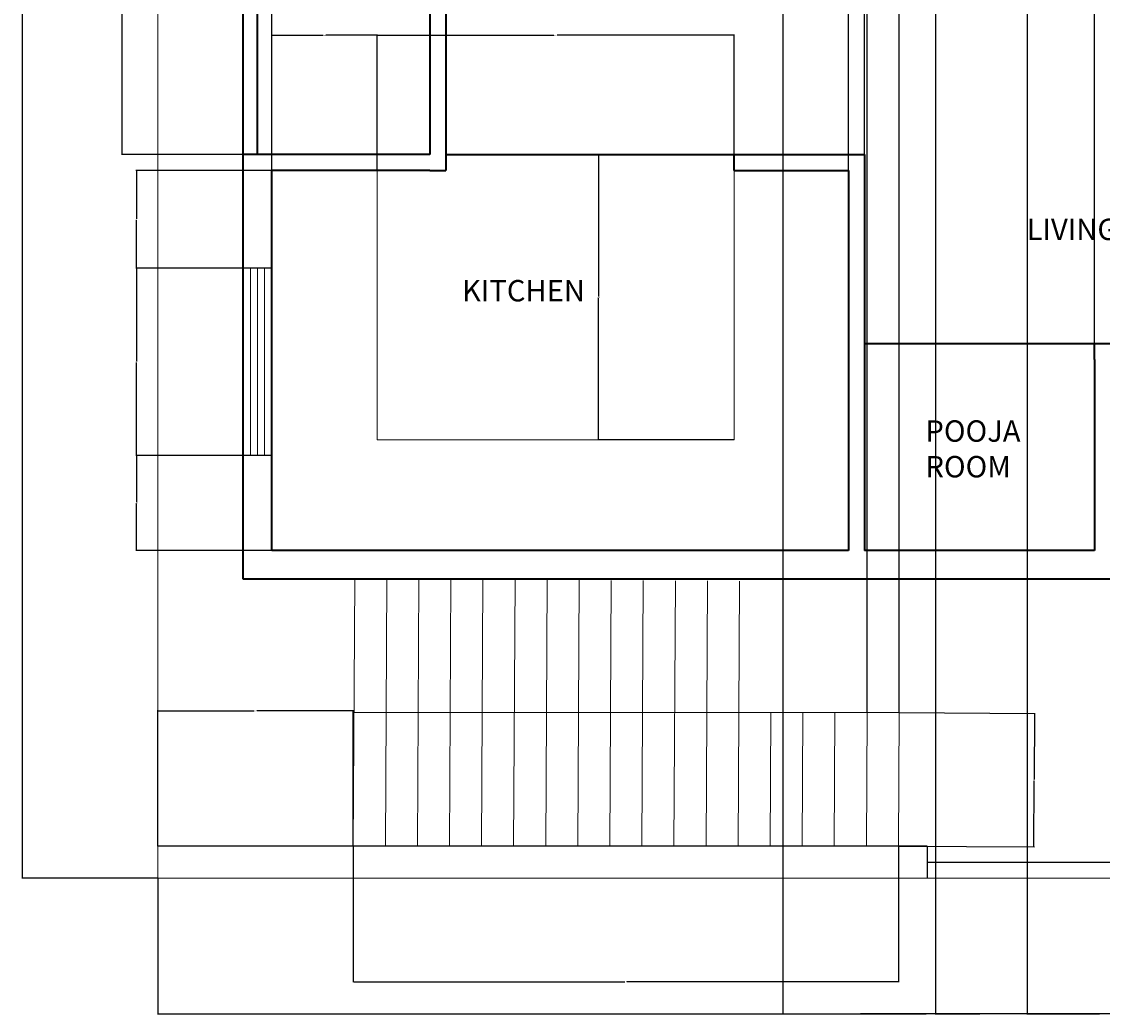
# Model space of a CAD drawing. Units: inches. Extents: x 4700 to 5209, y 8078 to 8754.
# Tile 1 of 5: x 4701 to 5004, y 8078 to 8356. Entities that reach past the tile are written whole.
import ezdxf

# ---------------------------------------------------------------- set-up
doc = ezdxf.new("R2010")
doc.units = ezdxf.units.IN
for name, color, linetype, lineweight in [('A-ANNO-DIMS', 2, 'Continuous', 18), ('A-AREA-IDEN', 7, 'Continuous', 18), ('A-FLOR', 7, 'Continuous', 25), ('A-FLOR-FIXT', 9, 'Continuous', 18), ('A-FLOR-STRS', 7, 'Continuous', 18), ('A-GLAZ', 4, 'Continuous', 18), ('A-WALL', 7, 'Continuous', 35), ('C-PROP', 8, 'Continuous', 18)]:
    doc.layers.add(name, color=color, linetype=linetype, lineweight=lineweight)
doc.styles.get("Standard").update_dxf_attribs({"font": 'arial.ttf'})
doc.dimstyles.get("Standard").update_dxf_attribs({"dimtxt": 0.18, "dimasz": 0.18, "dimexe": 0.18, "dimexo": 0.0625, "dimgap": 0.09, "dimtad": 0, "dimtih": 1, "dimtoh": 1, "dimdec": 4, "dimzin": 0, "dimdsep": 46, "dimtxsty": 'Standard', "dimcen": 0.09, "dimadec": 0, "dimazin": 0, "dimtfac": 1, "dimtdec": 4, "dimtofl": 0, "dimtmove": 0, "dimatfit": 3, "dimfxl": 1, "dimtolj": 1, "dimtzin": 0, "dimarcsym": 0})

# ---------------------------------------------------------------- blocks, each defined once
blk = doc.blocks.new('*D14')
at = {"layer": 'A-ANNO-DIMS', "color": 0, "lineweight": -2, "transparency": 16777216}
for p, q in [((4738.78, 8115.69), (4738.78, 8077.57)), ((5170.78, 8115.69), (5170.78, 8077.57)), ((4738.96, 8077.75), (4954.49, 8077.75)), ((5170.6, 8077.75), (4955.07, 8077.75))]:
    blk.add_line(p, q, dxfattribs=at)
at = {"layer": 'A-ANNO-DIMS', "color": 0, "transparency": 16777216}
for points in [[(4738.96, 8077.78), (4738.96, 8077.72), (4738.78, 8077.75)], [(5170.6, 8077.78), (5170.6, 8077.72), (5170.78, 8077.75)]]:
    blk.add_solid(points, dxfattribs=at)
at = {"layer": 'Defpoints', "color": 0, "transparency": 16777216}
for p in [(4738.78, 8115.75), (5170.78, 8115.75), (5170.78, 8077.75)]:
    blk.add_point(p, dxfattribs=at)
at = {"layer": 'A-ANNO-DIMS', "color": 0, "transparency": 16777216, "insert": (4954.78, 8077.75), "char_height": 0.18, "attachment_point": 5}
blk.add_mtext('\\A1;432', dxfattribs=at)
blk = doc.blocks.new('*D15')
at = {"layer": 'A-ANNO-DIMS', "color": 0, "lineweight": -2, "transparency": 16777216}
for p, q in [((4738.72, 8715.75), (4700.6, 8715.75)), ((4700.78, 8715.57), (4700.78, 8415.93)), ((4700.78, 8115.93), (4700.78, 8415.57)), ((4738.72, 8115.75), (4700.6, 8115.75))]:
    blk.add_line(p, q, dxfattribs=at)
at = {"layer": 'A-ANNO-DIMS', "color": 0, "transparency": 16777216}
for points in [[(4700.75, 8715.57), (4700.81, 8715.57), (4700.78, 8715.75)], [(4700.75, 8115.93), (4700.81, 8115.93), (4700.78, 8115.75)]]:
    blk.add_solid(points, dxfattribs=at)
at = {"layer": 'Defpoints', "color": 0, "transparency": 16777216}
for p in [(4700.78, 8715.75), (4738.78, 8715.75), (4738.78, 8115.75)]:
    blk.add_point(p, dxfattribs=at)
at = {"layer": 'A-ANNO-DIMS', "color": 0, "transparency": 16777216, "insert": (4700.78, 8415.75), "char_height": 0.18, "attachment_point": 5}
blk.add_mtext('\\A1;600', dxfattribs=at)
blk = doc.blocks.new('*D28')
at = {"layer": 'A-ANNO-DIMS', "color": 0, "lineweight": -2, "transparency": 16777216}
for p, q in [((4770.72, 8234.43), (4732.6, 8234.43)), ((4732.78, 8234.25), (4732.78, 8221.27)), ((4732.78, 8207.93), (4732.78, 8220.91)), ((4770.72, 8207.75), (4732.6, 8207.75))]:
    blk.add_line(p, q, dxfattribs=at)
at = {"layer": 'A-ANNO-DIMS', "color": 0, "transparency": 16777216}
for points in [[(4732.75, 8234.25), (4732.81, 8234.25), (4732.78, 8234.43)], [(4732.75, 8207.93), (4732.81, 8207.93), (4732.78, 8207.75)]]:
    blk.add_solid(points, dxfattribs=at)
at = {"layer": 'Defpoints', "color": 0, "transparency": 16777216}
for p in [(4732.78, 8234.43), (4770.78, 8234.43), (4770.78, 8207.75)]:
    blk.add_point(p, dxfattribs=at)
at = {"layer": 'A-ANNO-DIMS', "color": 0, "transparency": 16777216, "insert": (4732.78, 8221.09), "char_height": 0.18, "attachment_point": 5}
blk.add_mtext('\\A1;26.684', dxfattribs=at)
blk = doc.blocks.new('*D29')
at = {"layer": 'A-ANNO-DIMS', "color": 0, "lineweight": -2, "transparency": 16777216}
for p, q in [((4770.72, 8286.99), (4732.6, 8286.99)), ((4732.78, 8286.81), (4732.78, 8260.89)), ((4732.78, 8234.61), (4732.78, 8260.53)), ((4770.72, 8234.43), (4732.6, 8234.43))]:
    blk.add_line(p, q, dxfattribs=at)
at = {"layer": 'A-ANNO-DIMS', "color": 0, "transparency": 16777216}
for points in [[(4732.75, 8286.81), (4732.81, 8286.81), (4732.78, 8286.99)], [(4732.75, 8234.61), (4732.81, 8234.61), (4732.78, 8234.43)]]:
    blk.add_solid(points, dxfattribs=at)
at = {"layer": 'Defpoints', "color": 0, "transparency": 16777216}
for p in [(4732.78, 8286.99), (4770.78, 8286.99), (4770.78, 8234.43)]:
    blk.add_point(p, dxfattribs=at)
at = {"layer": 'A-ANNO-DIMS', "color": 0, "transparency": 16777216, "insert": (4732.78, 8260.71), "char_height": 0.18, "attachment_point": 5}
blk.add_mtext('\\A1;52.55', dxfattribs=at)
blk = doc.blocks.new('*D30')
at = {"layer": 'A-ANNO-DIMS', "color": 0, "lineweight": -2, "transparency": 16777216}
for p, q in [((4770.72, 8314.35), (4732.6, 8314.35)), ((4732.78, 8314.17), (4732.78, 8300.85)), ((4732.78, 8287.17), (4732.78, 8300.49)), ((4770.72, 8286.99), (4732.6, 8286.99))]:
    blk.add_line(p, q, dxfattribs=at)
at = {"layer": 'A-ANNO-DIMS', "color": 0, "transparency": 16777216}
for points in [[(4732.75, 8314.17), (4732.81, 8314.17), (4732.78, 8314.35)], [(4732.75, 8287.17), (4732.81, 8287.17), (4732.78, 8286.99)]]:
    blk.add_solid(points, dxfattribs=at)
at = {"layer": 'Defpoints', "color": 0, "transparency": 16777216}
for p in [(4732.78, 8314.35), (4770.78, 8314.35), (4770.78, 8286.99)]:
    blk.add_point(p, dxfattribs=at)
at = {"layer": 'A-ANNO-DIMS', "color": 0, "transparency": 16777216, "insert": (4732.78, 8300.67), "char_height": 0.18, "attachment_point": 5}
blk.add_mtext('\\A1;27.36', dxfattribs=at)
blk = doc.blocks.new('*D31')
at = {"layer": 'A-ANNO-DIMS', "color": 0, "lineweight": -2, "transparency": 16777216}
for p, q in [((4766.72, 8445.91), (4728.6, 8445.91)), ((4728.78, 8445.73), (4728.78, 8382.56)), ((4728.78, 8319.03), (4728.78, 8382.19)), ((4766.72, 8318.85), (4728.6, 8318.85))]:
    blk.add_line(p, q, dxfattribs=at)
at = {"layer": 'A-ANNO-DIMS', "color": 0, "transparency": 16777216}
for points in [[(4728.75, 8445.73), (4728.81, 8445.73), (4728.78, 8445.91)], [(4728.75, 8319.03), (4728.81, 8319.03), (4728.78, 8318.85)]]:
    blk.add_solid(points, dxfattribs=at)
at = {"layer": 'Defpoints', "color": 0, "transparency": 16777216}
for p in [(4728.78, 8445.91), (4766.78, 8445.91), (4766.78, 8318.85)]:
    blk.add_point(p, dxfattribs=at)
at = {"layer": 'A-ANNO-DIMS', "color": 0, "transparency": 16777216, "insert": (4728.78, 8382.38), "char_height": 0.18, "attachment_point": 5}
blk.add_mtext('\\A1;127.06', dxfattribs=at)
blk = doc.blocks.new('*D49')
at = {"layer": 'A-ANNO-DIMS', "color": 0, "lineweight": -2, "transparency": 16777216}
for p, q in [((4766.78, 8318.91), (4766.78, 8753.93)), ((4766.96, 8753.75), (4790.57, 8753.75)), ((4814.97, 8753.75), (4791.36, 8753.75)), ((4815.15, 8318.91), (4815.15, 8753.93))]:
    blk.add_line(p, q, dxfattribs=at)
at = {"layer": 'A-ANNO-DIMS', "color": 0, "transparency": 16777216}
for points in [[(4766.96, 8753.78), (4766.96, 8753.72), (4766.78, 8753.75)], [(4814.97, 8753.78), (4814.97, 8753.72), (4815.15, 8753.75)]]:
    blk.add_solid(points, dxfattribs=at)
at = {"layer": 'Defpoints', "color": 0, "transparency": 16777216}
for p in [(4815.15, 8753.75), (4766.78, 8318.85), (4815.15, 8318.85)]:
    blk.add_point(p, dxfattribs=at)
at = {"layer": 'A-ANNO-DIMS', "color": 0, "transparency": 16777216, "insert": (4790.96, 8753.75), "char_height": 0.18, "attachment_point": 5}
blk.add_mtext('\\A1;48.37', dxfattribs=at)
blk = doc.blocks.new('*D51')
at = {"layer": 'A-ANNO-DIMS', "color": 0, "lineweight": -2, "transparency": 16777216}
for p, q in [((4770.78, 8207.81), (4770.78, 8753.93)), ((4770.96, 8753.75), (4851.26, 8753.75)), ((4932.47, 8753.75), (4852.17, 8753.75)), ((4932.65, 8207.81), (4932.65, 8753.93))]:
    blk.add_line(p, q, dxfattribs=at)
at = {"layer": 'A-ANNO-DIMS', "color": 0, "transparency": 16777216}
for points in [[(4770.96, 8753.78), (4770.96, 8753.72), (4770.78, 8753.75)], [(4932.47, 8753.78), (4932.47, 8753.72), (4932.65, 8753.75)]]:
    blk.add_solid(points, dxfattribs=at)
at = {"layer": 'Defpoints', "color": 0, "transparency": 16777216}
for p in [(4932.65, 8753.75), (4770.78, 8207.75), (4932.65, 8207.75)]:
    blk.add_point(p, dxfattribs=at)
at = {"layer": 'A-ANNO-DIMS', "color": 0, "transparency": 16777216, "insert": (4851.71, 8753.75), "char_height": 0.18, "attachment_point": 5}
blk.add_mtext('\\A1;161.87', dxfattribs=at)
blk = doc.blocks.new('*D52')
at = {"layer": 'A-ANNO-DIMS', "color": 0, "lineweight": -2, "transparency": 16777216}
for p, q in [((4800.37, 8314.41), (4800.37, 8352.53)), ((4800.55, 8352.35), (4850, 8352.35)), ((4900.35, 8352.35), (4850.91, 8352.35)), ((4900.53, 8314.41), (4900.53, 8352.53))]:
    blk.add_line(p, q, dxfattribs=at)
at = {"layer": 'A-ANNO-DIMS', "color": 0, "transparency": 16777216}
for points in [[(4800.55, 8352.38), (4800.55, 8352.32), (4800.37, 8352.35)], [(4900.35, 8352.38), (4900.35, 8352.32), (4900.53, 8352.35)]]:
    blk.add_solid(points, dxfattribs=at)
at = {"layer": 'Defpoints', "color": 0, "transparency": 16777216}
for p in [(4900.53, 8352.35), (4800.37, 8314.35), (4900.53, 8314.35)]:
    blk.add_point(p, dxfattribs=at)
at = {"layer": 'A-ANNO-DIMS', "color": 0, "transparency": 16777216, "insert": (4850.45, 8352.35), "char_height": 0.18, "attachment_point": 5}
blk.add_mtext('\\A1;100.16', dxfattribs=at)
blk = doc.blocks.new('*D53')
at = {"layer": 'A-ANNO-DIMS', "color": 0, "lineweight": -2, "transparency": 16777216}
for p, q in [((4770.78, 8314.41), (4770.78, 8352.53)), ((4770.96, 8352.35), (4785.18, 8352.35)), ((4800.19, 8352.35), (4785.97, 8352.35)), ((4800.37, 8314.41), (4800.37, 8352.53))]:
    blk.add_line(p, q, dxfattribs=at)
at = {"layer": 'A-ANNO-DIMS', "color": 0, "transparency": 16777216}
for points in [[(4770.96, 8352.38), (4770.96, 8352.32), (4770.78, 8352.35)], [(4800.19, 8352.38), (4800.19, 8352.32), (4800.37, 8352.35)]]:
    blk.add_solid(points, dxfattribs=at)
at = {"layer": 'Defpoints', "color": 0, "transparency": 16777216}
for p in [(4800.37, 8352.35), (4770.78, 8314.35), (4800.37, 8314.35)]:
    blk.add_point(p, dxfattribs=at)
at = {"layer": 'A-ANNO-DIMS', "color": 0, "transparency": 16777216, "insert": (4785.58, 8352.35), "char_height": 0.18, "attachment_point": 5}
blk.add_mtext('\\A1;29.59', dxfattribs=at)
blk = doc.blocks.new('*D54')
at = {"layer": 'A-ANNO-DIMS', "color": 0, "lineweight": -2, "transparency": 16777216}
for p, q in [((4900.47, 8318.85), (4862.35, 8318.85)), ((4862.53, 8318.67), (4862.53, 8279.01)), ((4862.53, 8238.98), (4862.53, 8278.64)), ((4900.47, 8238.8), (4862.35, 8238.8))]:
    blk.add_line(p, q, dxfattribs=at)
at = {"layer": 'A-ANNO-DIMS', "color": 0, "transparency": 16777216}
for points in [[(4862.5, 8318.67), (4862.56, 8318.67), (4862.53, 8318.85)], [(4862.5, 8238.98), (4862.56, 8238.98), (4862.53, 8238.8)]]:
    blk.add_solid(points, dxfattribs=at)
at = {"layer": 'Defpoints', "color": 0, "transparency": 16777216}
for p in [(4862.53, 8318.85), (4900.53, 8318.85), (4900.53, 8238.8)]:
    blk.add_point(p, dxfattribs=at)
at = {"layer": 'A-ANNO-DIMS', "color": 0, "transparency": 16777216, "insert": (4862.53, 8278.83), "char_height": 0.18, "attachment_point": 5}
blk.add_mtext('\\A1;80.05', dxfattribs=at)
blk = doc.blocks.new('*D55')
at = {"layer": 'A-ANNO-DIMS', "color": 0, "lineweight": -2, "transparency": 16777216}
for p, q in [((4937.15, 8207.81), (4937.15, 8753.93)), ((4937.33, 8753.75), (4969.02, 8753.75)), ((5001.49, 8753.75), (4969.8, 8753.75)), ((5001.67, 8207.81), (5001.67, 8753.93))]:
    blk.add_line(p, q, dxfattribs=at)
at = {"layer": 'A-ANNO-DIMS', "color": 0, "transparency": 16777216}
for points in [[(4937.33, 8753.78), (4937.33, 8753.72), (4937.15, 8753.75)], [(5001.49, 8753.78), (5001.49, 8753.72), (5001.67, 8753.75)]]:
    blk.add_solid(points, dxfattribs=at)
at = {"layer": 'Defpoints', "color": 0, "transparency": 16777216}
for p in [(5001.67, 8753.75), (4937.15, 8207.75), (5001.67, 8207.75)]:
    blk.add_point(p, dxfattribs=at)
at = {"layer": 'A-ANNO-DIMS', "color": 0, "transparency": 16777216, "insert": (4969.41, 8753.75), "char_height": 0.18, "attachment_point": 5}
blk.add_mtext('\\A1;64.53', dxfattribs=at)
blk = doc.blocks.new('*D60')
at = {"layer": 'A-ANNO-DIMS', "color": 0, "lineweight": -2, "transparency": 16777216}
for p, q in [((4793.67, 8124.69), (4793.67, 8086.57)), ((4946.67, 8124.69), (4946.67, 8086.57)), ((4793.85, 8086.75), (4869.89, 8086.75)), ((4946.49, 8086.75), (4870.45, 8086.75))]:
    blk.add_line(p, q, dxfattribs=at)
at = {"layer": 'A-ANNO-DIMS', "color": 0, "transparency": 16777216}
for points in [[(4793.85, 8086.78), (4793.85, 8086.72), (4793.67, 8086.75)], [(4946.49, 8086.78), (4946.49, 8086.72), (4946.67, 8086.75)]]:
    blk.add_solid(points, dxfattribs=at)
at = {"layer": 'Defpoints', "color": 0, "transparency": 16777216}
for p in [(4793.67, 8124.75), (4946.67, 8124.75), (4793.67, 8086.75)]:
    blk.add_point(p, dxfattribs=at)
at = {"layer": 'A-ANNO-DIMS', "color": 0, "transparency": 16777216, "insert": (4870.17, 8086.75), "char_height": 0.18, "attachment_point": 5}
blk.add_mtext('\\A1;153', dxfattribs=at)
blk = doc.blocks.new('*D61')
at = {"layer": 'A-ANNO-DIMS', "color": 0, "lineweight": -2, "transparency": 16777216}
for p, q in [((4946.93, 8162.25), (4985.05, 8162.05)), ((4984.87, 8161.87), (4984.77, 8143.48)), ((4984.68, 8124.73), (4984.77, 8143.12)), ((4946.74, 8124.75), (4984.85, 8124.55))]:
    blk.add_line(p, q, dxfattribs=at)
at = {"layer": 'A-ANNO-DIMS', "color": 0, "transparency": 16777216}
for points in [[(4984.84, 8161.87), (4984.9, 8161.87), (4984.87, 8162.05)], [(4984.65, 8124.73), (4984.71, 8124.73), (4984.67, 8124.55)]]:
    blk.add_solid(points, dxfattribs=at)
at = {"layer": 'Defpoints', "color": 0, "transparency": 16777216}
for p in [(4946.87, 8162.25), (4946.67, 8124.75), (4984.67, 8124.55)]:
    blk.add_point(p, dxfattribs=at)
at = {"layer": 'A-ANNO-DIMS', "color": 0, "transparency": 16777216, "insert": (4984.77, 8143.3), "char_height": 0.18, "attachment_point": 5}
blk.add_mtext('\\A1;37.5', dxfattribs=at)
blk = doc.blocks.new('*D62')
at = {"layer": 'A-ANNO-DIMS', "color": 0, "lineweight": -2, "transparency": 16777216}
for p, q in [((4937.87, 8162.31), (4937.87, 8753.93)), ((4938.05, 8753.75), (4942.22, 8753.75)), ((4946.69, 8753.75), (4942.52, 8753.75)), ((4946.87, 8162.31), (4946.87, 8753.93))]:
    blk.add_line(p, q, dxfattribs=at)
at = {"layer": 'A-ANNO-DIMS', "color": 0, "transparency": 16777216}
for points in [[(4938.05, 8753.78), (4938.05, 8753.72), (4937.87, 8753.75)], [(4946.69, 8753.78), (4946.69, 8753.72), (4946.87, 8753.75)]]:
    blk.add_solid(points, dxfattribs=at)
at = {"layer": 'Defpoints', "color": 0, "transparency": 16777216}
for p in [(4946.87, 8753.75), (4937.87, 8162.25), (4946.87, 8162.25)]:
    blk.add_point(p, dxfattribs=at)
at = {"layer": 'A-ANNO-DIMS', "color": 0, "transparency": 16777216, "insert": (4942.37, 8753.75), "char_height": 0.18, "attachment_point": 5}
blk.add_mtext('\\A1;9', dxfattribs=at)
blk = doc.blocks.new('*D63')
at = {"layer": 'A-ANNO-DIMS', "color": 0, "lineweight": -2, "transparency": 16777216}
for p, q in [((4914.2, 8523.69), (4914.2, 8077.57)), ((4957.05, 8523.69), (4957.05, 8077.57)), ((4914.38, 8077.75), (4935.23, 8077.75)), ((4956.87, 8077.75), (4936.02, 8077.75))]:
    blk.add_line(p, q, dxfattribs=at)
at = {"layer": 'A-ANNO-DIMS', "color": 0, "transparency": 16777216}
for points in [[(4914.38, 8077.78), (4914.38, 8077.72), (4914.2, 8077.75)], [(4956.87, 8077.78), (4956.87, 8077.72), (4957.05, 8077.75)]]:
    blk.add_solid(points, dxfattribs=at)
at = {"layer": 'Defpoints', "color": 0, "transparency": 16777216}
for p in [(4914.2, 8523.75), (4957.05, 8523.75), (4957.05, 8077.75)]:
    blk.add_point(p, dxfattribs=at)
at = {"layer": 'A-ANNO-DIMS', "color": 0, "transparency": 16777216, "insert": (4935.63, 8077.75), "char_height": 0.18, "attachment_point": 5}
blk.add_mtext('\\A1;42.85', dxfattribs=at)
blk = doc.blocks.new('*D64')
at = {"layer": 'A-ANNO-DIMS', "color": 0, "lineweight": -2, "transparency": 16777216}
for p, q in [((4982.78, 8523.69), (4982.78, 8077.57)), ((5024.22, 8523.69), (5024.22, 8077.57)), ((4982.96, 8077.75), (5003.1, 8077.75)), ((5024.04, 8077.75), (5003.9, 8077.75))]:
    blk.add_line(p, q, dxfattribs=at)
at = {"layer": 'A-ANNO-DIMS', "color": 0, "transparency": 16777216}
for points in [[(4982.96, 8077.78), (4982.96, 8077.72), (4982.78, 8077.75)], [(5024.04, 8077.78), (5024.04, 8077.72), (5024.22, 8077.75)]]:
    blk.add_solid(points, dxfattribs=at)
at = {"layer": 'Defpoints', "color": 0, "transparency": 16777216}
for p in [(4982.78, 8523.75), (5024.22, 8523.75), (5024.22, 8077.75)]:
    blk.add_point(p, dxfattribs=at)
at = {"layer": 'A-ANNO-DIMS', "color": 0, "transparency": 16777216, "insert": (5003.5, 8077.75), "char_height": 0.18, "attachment_point": 5}
blk.add_mtext('\\A1;41.44', dxfattribs=at)
blk = doc.blocks.new('*D65')
at = {"layer": 'A-ANNO-DIMS', "color": 0, "lineweight": -2, "transparency": 16777216}
for p, q in [((4957.05, 8523.69), (4957.05, 8077.57)), ((4982.78, 8523.69), (4982.78, 8077.57)), ((4957.23, 8077.75), (4969.52, 8077.75)), ((4982.6, 8077.75), (4970.31, 8077.75))]:
    blk.add_line(p, q, dxfattribs=at)
at = {"layer": 'A-ANNO-DIMS', "color": 0, "transparency": 16777216}
for points in [[(4957.23, 8077.78), (4957.23, 8077.72), (4957.05, 8077.75)], [(4982.6, 8077.78), (4982.6, 8077.72), (4982.78, 8077.75)]]:
    blk.add_solid(points, dxfattribs=at)
at = {"layer": 'Defpoints', "color": 0, "transparency": 16777216}
for p in [(4957.05, 8523.75), (4982.78, 8523.75), (4982.78, 8077.75)]:
    blk.add_point(p, dxfattribs=at)
at = {"layer": 'A-ANNO-DIMS', "color": 0, "transparency": 16777216, "insert": (4969.91, 8077.75), "char_height": 0.18, "attachment_point": 5}
blk.add_mtext('\\A1;25.73', dxfattribs=at)
blk = doc.blocks.new('*D72')
at = {"layer": 'A-ANNO-DIMS', "color": 0, "lineweight": -2, "transparency": 16777216}
for p, q in [((4738.78, 8124.81), (4738.78, 8162.93)), ((4738.96, 8162.75), (4765.83, 8162.75)), ((4793.49, 8162.75), (4766.62, 8162.75)), ((4793.67, 8124.81), (4793.67, 8162.93))]:
    blk.add_line(p, q, dxfattribs=at)
at = {"layer": 'A-ANNO-DIMS', "color": 0, "transparency": 16777216}
for points in [[(4738.96, 8162.78), (4738.96, 8162.72), (4738.78, 8162.75)], [(4793.49, 8162.78), (4793.49, 8162.72), (4793.67, 8162.75)]]:
    blk.add_solid(points, dxfattribs=at)
at = {"layer": 'Defpoints', "color": 0, "transparency": 16777216}
for p in [(4793.67, 8162.75), (4738.78, 8124.75), (4793.67, 8124.75)]:
    blk.add_point(p, dxfattribs=at)
at = {"layer": 'A-ANNO-DIMS', "color": 0, "transparency": 16777216, "insert": (4766.23, 8162.75), "char_height": 0.18, "attachment_point": 5}
blk.add_mtext('\\A1;54.89', dxfattribs=at)

msp = doc.modelspace()

# ---------------------------------------------------------------- linework, layer by layer
at = {"layer": 'A-FLOR'}
for p, q in [((4954.7803, 8124.7503), (4738.7803, 8124.7503)), ((4954.7803, 8124.7503), (4954.7803, 8115.7503)), ((4954.7803, 8120.2503), (5140.9801, 8120.2503))]:
    msp.add_line(p, q, dxfattribs=at)
at = {"layer": 'A-FLOR-FIXT'}
for p, q in [((4800.372, 8314.3479), (4800.372, 8238.8027)), ((4900.5332, 8238.8027), (4900.5332, 8314.3479)), ((4800.372, 8238.8027), (4900.5332, 8238.8027))]:
    msp.add_line(p, q, dxfattribs=at)
at = {"layer": 'A-FLOR-STRS'}
for p, q in [((4794.0633, 8199.7503), (4793.6728, 8124.7503)), ((4803.0632, 8199.7035), (4802.6729, 8124.7503)), ((4812.0631, 8199.6566), (4811.673, 8124.7503)), ((4821.0629, 8199.6097), (4820.6731, 8124.7503)), ((4830.0628, 8199.5629), (4829.6733, 8124.7503)), ((4839.0627, 8199.516), (4838.6734, 8124.7503)), ((4848.0626, 8199.4692), (4847.6735, 8124.7503)), ((4857.0625, 8199.4223), (4856.6736, 8124.7503)), ((4866.0623, 8199.3754), (4865.6737, 8124.7503)), ((4875.0622, 8199.3286), (4874.6739, 8124.7503)), ((4884.0621, 8199.2817), (4883.674, 8124.7503)), ((4893.062, 8199.2348), (4892.6741, 8124.7503)), ((4902.0618, 8199.188), (4901.6742, 8124.7503)), ((4793.868, 8162.2503), (4946.8701, 8162.2503)), ((4910.8696, 8162.2503), (4910.6744, 8124.7503)), ((4919.8697, 8162.2503), (4919.6745, 8124.7503)), ((4928.8699, 8162.2503), (4928.6746, 8124.7503)), ((4937.87, 8162.2503), (4937.6747, 8124.7503)), ((4946.8701, 8162.2503), (4946.6748, 8124.7503))]:
    msp.add_line(p, q, dxfattribs=at)
at = {"layer": 'A-GLAZ'}
for p, q in [((4764.8543, 8286.987), (4764.8543, 8234.4346)), ((4766.7803, 8286.987), (4766.7803, 8234.4346)), ((4768.7397, 8286.987), (4768.7397, 8234.4346))]:
    msp.add_line(p, q, dxfattribs=at)
msp.add_lwpolyline([(4762.7803, 8286.987), (4770.7803, 8286.987), (4770.7803, 8234.4346), (4762.7803, 8234.4346)], close=True, dxfattribs=at)
at = {"layer": 'A-WALL'}
for p, q in [((4762.7803, 8199.7503), (4762.7803, 8691.7503)), ((4766.7803, 8318.8479), (4766.7803, 8445.9056)), ((4815.1488, 8445.9056), (4815.1488, 8318.8479)), ((4819.6488, 8445.9056), (4819.6488, 8318.8479)), ((4770.7803, 8318.8479), (4762.7803, 8318.8479)), ((4815.1488, 8318.8479), (4770.7803, 8318.8479)), ((4819.6488, 8318.8479), (4937.1464, 8318.8479)), ((4819.6488, 8318.8479), (4819.6488, 8314.3479)), ((4900.5332, 8314.3479), (4900.5332, 8318.8479)), ((4937.1464, 8318.8479), (4937.1464, 8265.8608)), ((4770.7803, 8207.7503), (4770.7803, 8314.3479)), ((4815.1488, 8314.3479), (4770.7803, 8314.3479)), ((4815.1488, 8314.3479), (4819.6488, 8314.3479)), ((4900.5332, 8314.3479), (4932.6464, 8314.3479)), ((4932.6464, 8314.3479), (4932.6464, 8207.7503)), ((4937.1464, 8265.8608), (5006.1744, 8265.8608)), ((4937.1464, 8265.8608), (4937.1464, 8261.3608)), ((5001.6744, 8261.3608), (5001.6744, 8265.8608)), ((4937.1464, 8261.3608), (4937.1464, 8207.7503)), ((5001.6744, 8261.3608), (5001.6744, 8207.7503)), ((4932.6464, 8207.7503), (4770.7803, 8207.7503)), ((5001.6744, 8207.7503), (4937.1464, 8207.7503)), ((5146.7803, 8199.7503), (4762.7803, 8199.7503))]:
    msp.add_line(p, q, dxfattribs=at)
at = {"layer": 'C-PROP'}
for p, q in [((4738.7803, 8115.7503), (4738.7803, 8715.7503)), ((5170.7803, 8115.7503), (4738.7803, 8115.7503))]:
    msp.add_line(p, q, dxfattribs=at)

# ---------------------------------------------------------------- texts
at = {"layer": 'A-AREA-IDEN', "char_height": 6, "attachment_point": 1}
for s, width, insert in [('\\pxi-3,l4,t4;LIVING HALL ', 80.039779, (4976.653, 8300.8555)), ('KITCHEN', 51.756341, (4824.1773, 8283.6591)), ('POOJA ROOM ', 51.756341, (4954.2641, 8244.2741))]:
    msp.add_mtext_dynamic_manual_height_columns(s, width=width, gutter_width=12.5, heights=[0], dxfattribs=dict(at, insert=insert))

# ---------------------------------------------------------------- dimensions: what is measured, and where the dimension line sits
at = {"layer": 'A-ANNO-DIMS'}
for base, p1, p2, override, picture, middle in [((4815.1488, 8753.7503), (4766.7803, 8318.8479), (4815.1488, 8318.8479), {"dimdec": 2, "dimlfac": 1, "dimrnd": 0, "dimzin": 0, "dimdsep": 46, "dimlunit": 2}, '*D49', (4790.9646, 8753.7503)), ((4932.6464, 8753.7503), (4770.7803, 8207.7503), (4932.6464, 8207.7503), {"dimdec": 2, "dimlfac": 1, "dimrnd": 0, "dimzin": 0, "dimdsep": 46, "dimlunit": 2}, '*D51', (4851.7134, 8753.7503)), ((5001.6744, 8753.7503), (4937.1464, 8207.7503), (5001.6744, 8207.7503), {"dimdec": 2, "dimlfac": 1, "dimrnd": 0, "dimzin": 0, "dimdsep": 46, "dimlunit": 2}, '*D55', (4969.4104, 8753.7503)), ((4946.8701, 8753.7503), (4937.87, 8162.2503), (4946.8701, 8162.2503), {"dimdec": 0, "dimlfac": 1, "dimrnd": 0, "dimzin": 0, "dimdsep": 46, "dimlunit": 2}, '*D62', (4942.3701, 8753.7503)), ((4957.0498, 8077.7503), (4914.2028, 8523.7503), (4957.0498, 8523.7503), {"dimdec": 2, "dimlfac": 1, "dimrnd": 0, "dimzin": 0, "dimdsep": 46, "dimlunit": 2}, '*D63', (4935.6263, 8077.7503)), ((4982.778, 8077.7503), (4957.0498, 8523.7503), (4982.778, 8523.7503), {"dimdec": 2, "dimlfac": 1, "dimrnd": 0, "dimzin": 0, "dimdsep": 46, "dimlunit": 2}, '*D65', (4969.9139, 8077.7503)), ((5024.2192, 8077.7503), (4982.778, 8523.7503), (5024.2192, 8523.7503), {"dimdec": 2, "dimlfac": 1, "dimrnd": 0, "dimzin": 0, "dimdsep": 46, "dimlunit": 2}, '*D64', (5003.4986, 8077.7503)), ((4800.372, 8352.3479), (4770.7803, 8314.3479), (4800.372, 8314.3479), {"dimdec": 2, "dimlfac": 1, "dimrnd": 0, "dimzin": 0, "dimdsep": 46, "dimlunit": 2}, '*D53', (4785.5761, 8352.3479)), ((4900.5332, 8352.3479), (4800.372, 8314.3479), (4900.5332, 8314.3479), {"dimdec": 2, "dimlfac": 1, "dimrnd": 0, "dimzin": 0, "dimdsep": 46, "dimlunit": 2}, '*D52', (4850.4526, 8352.3479)), ((4793.6728, 8162.7503), (4738.7803, 8124.7503), (4793.6728, 8124.7503), {"dimdec": 2, "dimlfac": 1, "dimrnd": 0, "dimzin": 0, "dimdsep": 46, "dimlunit": 2}, '*D72', (4766.2265, 8162.7503)), ((5170.7803, 8077.7503), (4738.7803, 8115.7503), (5170.7803, 8115.7503), {"dimdec": 0, "dimlfac": 1, "dimrnd": 0, "dimzin": 0, "dimdsep": 46, "dimlunit": 2}, '*D14', (4954.7803, 8077.7503))]:
    dim = msp.add_linear_dim(base=base, p1=p1, p2=p2, dimstyle='Standard', override=override, dxfattribs=at)
    dim.commit()
    dim.dimension.update_dxf_attribs({"geometry": picture, "text_midpoint": middle})
for base, p1, p2, angle, override, picture, middle in [((4700.7803, 8715.7503), (4738.7803, 8115.7503), (4738.7803, 8715.7503), 90, {"dimdec": 0, "dimlfac": 1, "dimrnd": 0, "dimzin": 0, "dimdsep": 46, "dimlunit": 2}, '*D15', (4700.7803, 8415.7503)), ((4728.7803, 8445.9056), (4766.7803, 8318.8479), (4766.7803, 8445.9056), 90, {"dimdec": 2, "dimlfac": 1, "dimrnd": 0, "dimzin": 0, "dimdsep": 46, "dimlunit": 2}, '*D31', (4728.7803, 8382.3768)), ((4862.5332, 8318.8479), (4900.5332, 8238.8027), (4900.5332, 8318.8479), 90, {"dimdec": 2, "dimlfac": 1, "dimrnd": 0, "dimzin": 0, "dimdsep": 46, "dimlunit": 2}, '*D54', (4862.5332, 8278.8253)), ((4732.7803, 8314.3479), (4770.7803, 8286.987), (4770.7803, 8314.3479), 90, {"dimdec": 2, "dimlfac": 1, "dimrnd": 0, "dimzin": 0, "dimdsep": 46, "dimlunit": 2}, '*D30', (4732.7803, 8300.6674)), ((4732.7803, 8286.987), (4770.7803, 8234.4346), (4770.7803, 8286.987), 90, {"dimdec": 2, "dimlfac": 1, "dimrnd": 0, "dimzin": 0, "dimdsep": 46, "dimlunit": 2}, '*D29', (4732.7803, 8260.7108)), ((4732.7803, 8234.4346), (4770.7803, 8207.7503), (4770.7803, 8234.4346), 90, {"dimdec": 3, "dimlfac": 1, "dimrnd": 0, "dimzin": 0, "dimdsep": 46, "dimlunit": 2}, '*D28', (4732.7803, 8221.0925)), ((4984.6743, 8124.5525), (4946.8701, 8162.2503), (4946.6748, 8124.7503), 269.701657, {"dimdec": 1, "dimlfac": 1, "dimrnd": 0, "dimzin": 0, "dimdsep": 46, "dimlunit": 2}, '*D61', (4984.772, 8143.3025)), ((4793.6728, 8086.7503), (4946.6748, 8124.7503), (4793.6728, 8124.7503), 180, {"dimdec": 0, "dimlfac": 1, "dimrnd": 0, "dimzin": 0, "dimdsep": 46, "dimlunit": 2}, '*D60', (4870.1738, 8086.7503))]:
    dim = msp.add_linear_dim(base=base, p1=p1, p2=p2, angle=angle, dimstyle='Standard', override=override, dxfattribs=at)
    dim.commit()
    dim.dimension.update_dxf_attribs({"geometry": picture, "text_midpoint": middle})

doc.saveas('drawing.dxf')
